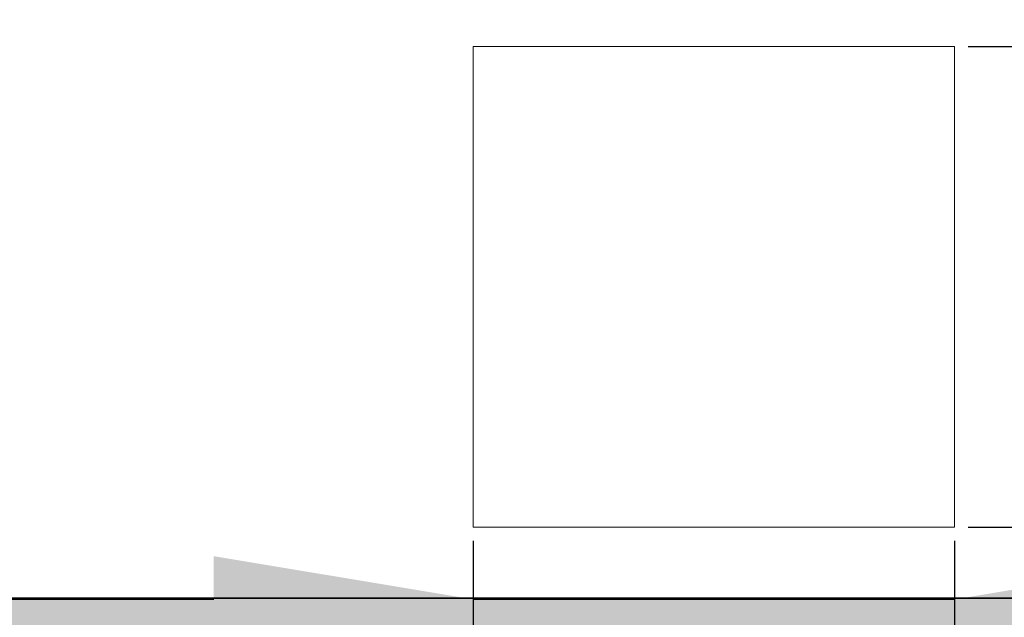
# Model space of a CAD drawing. Units: inches. Extents: x 2083 to 3317, y 1141 to 2115.
# Tile 238 of 256: x 3068 to 3114, y 1271 to 1299. Entities that reach past the tile are written whole.
import ezdxf

# ---------------------------------------------------------------- set-up
doc = ezdxf.new("R2010")
doc.units = ezdxf.units.IN
for name, color, linetype, lineweight in [('A-ANNO-DIMS', 2, 'Continuous', 18), ('A-FURN', 8, 'Continuous', 18), ('A-WALL', 7, 'Continuous', 35)]:
    doc.layers.add(name, color=color, linetype=linetype, lineweight=lineweight)
doc.layers.add('A-WALL-PATT', color=251, linetype='Continuous', lineweight=13, true_color=0x636466)
doc.styles.get("Standard").update_dxf_attribs({"font": 'arial.ttf'})
doc.dimstyles.new('ISO-25', dxfattribs={"dimtxt": 12, "dimasz": 12, "dimexe": 1.25, "dimexo": 0.625, "dimtad": 1, "dimlunit": 3, "dimtxsty": 'Standard', "dimcen": 2.5, "dimadec": 0, "dimazin": 0, "dimtfac": 1, "dimtmove": 0, "dimatfit": 3, "dimfxl": 1, "dimarcsym": 0})

# ---------------------------------------------------------------- blocks, each defined once
blk = doc.blocks.new('NIGHTSTAND-COMPACT')
blk.add_lwpolyline([(22.254, 22.255), (22.254, 0), (0, 0), (0, 22.255)], close=True)
blk = doc.blocks.new('*D26')
at = {"layer": 'A-ANNO-DIMS', "color": 0, "lineweight": -2, "transparency": 16777216}
for p, q in [((3088.986, 1274.915), (3088.986, 1270.952)), ((3111.24, 1274.915), (3111.24, 1270.952)), ((3076.986, 1272.202), (2840.262, 1272.202)), ((3111.24, 1272.202), (3088.986, 1272.202)), ((3123.24, 1272.202), (3135.24, 1272.202))]:
    blk.add_line(p, q, dxfattribs=at)
at = {"layer": 'A-ANNO-DIMS', "color": 0, "transparency": 16777216}
for points in [[(3076.986, 1274.202), (3076.986, 1270.202), (3088.986, 1272.202)], [(3123.24, 1274.202), (3123.24, 1270.202), (3111.24, 1272.202)]]:
    blk.add_solid(points, dxfattribs=at)
at = {"layer": 'Defpoints', "color": 0, "transparency": 16777216}
for p in [(3088.986, 1275.54), (3111.24, 1275.54), (3088.986, 1272.202)]:
    blk.add_point(p, dxfattribs=at)
at = {"layer": 'A-ANNO-DIMS', "color": 0, "transparency": 16777216, "insert": (2952.624, 1279.032), "char_height": 12, "attachment_point": 5}
blk.add_mtext('NIGHTSTAND 1\'-10 1/2" TYP.', dxfattribs=at)
blk = doc.blocks.new('*D27')
at = {"layer": 'A-ANNO-DIMS', "color": 0, "lineweight": -2, "transparency": 16777216}
for p, q in [((3114.578, 1309.794), (3114.578, 1321.794)), ((3111.865, 1297.794), (3115.828, 1297.794)), ((3114.578, 1297.794), (3114.578, 1275.54)), ((3111.865, 1275.54), (3115.828, 1275.54)), ((3114.578, 1263.54), (3114.578, 1140.989))]:
    blk.add_line(p, q, dxfattribs=at)
at = {"layer": 'A-ANNO-DIMS', "color": 0, "transparency": 16777216}
for points in [[(3112.578, 1309.794), (3116.578, 1309.794), (3114.578, 1297.794)], [(3112.578, 1263.54), (3116.578, 1263.54), (3114.578, 1275.54)]]:
    blk.add_solid(points, dxfattribs=at)
at = {"layer": 'Defpoints', "color": 0, "transparency": 16777216}
for p in [(3111.24, 1297.794), (3111.24, 1275.54), (3114.578, 1275.54)]:
    blk.add_point(p, dxfattribs=at)
at = {"layer": 'A-ANNO-DIMS', "color": 0, "transparency": 16777216, "insert": (3107.749, 1196.264), "char_height": 12, "attachment_point": 5, "rotation": 90}
blk.add_mtext('1\'-10 1/2" TYP.', dxfattribs=at)

msp = doc.modelspace()

# ---------------------------------------------------------------- hatches: boundary and pattern name
at = {"layer": 'A-WALL-PATT'}
h = msp.add_hatch(color=256, dxfattribs=at)
h.dxf.hatch_style = 1
h.paths.add_polyline_path([(3126.96, 2020.761), (2748.96, 2020.761), (2604.96, 2020.761), (2226.96, 2020.761), (2226.96, 1702.761), (2466.96, 1702.761), (2466.96, 1582.761), (2418.96, 1582.761), (2418.96, 1477.761), (2226.96, 1477.761), (2226.96, 1263.261), (2544.96, 1263.261), (2544.96, 1411.761), (2604.96, 1411.761), (2685.96, 1411.761), (2685.96, 1420.761), (2604.96, 1420.761), (2604.96, 1573.761), (2604.96, 1702.761), (2604.96, 2011.761), (2748.96, 2011.761), (2748.96, 1702.761), (2862.96, 1702.761), (2862.96, 1621.761), (2871.96, 1621.761), (2871.96, 1702.761), (2883.96, 1702.761), (2883.96, 1706.939, -0.026459), (2883.96, 1711.761), (2757.96, 1711.761), (2757.96, 1807.761), (2787.96, 1807.761), (2787.96, 1812.261), (2757.96, 1812.261), (2757.96, 2011.761), (2877.96, 2011.761), (2877.96, 1812.261), (2847.96, 1812.261), (2847.96, 1807.761), (2889.836, 1807.761), (2889.836, 1812.261), (2882.46, 1812.261), (2882.46, 2011.761), (3117.96, 2011.761), (3117.96, 1812.261), (2937.836, 1812.261), (2937.836, 1807.761), (2995.71, 1807.761), (2995.71, 1796.118), (3000.21, 1796.118), (3000.21, 1807.761), (3117.96, 1807.761), (3117.96, 1711.761), (3000.21, 1711.761), (3000.21, 1760.118), (2998.573, 1760.118, -0.020711), (2995.71, 1760.118), (2995.71, 1711.761), (2931.96, 1711.761), (2931.96, 1702.761), (3126.96, 1702.761)])
h.paths.add_polyline_path([(2471.46, 2011.761), (2471.46, 1810.011), (2462.717, 1810.011), (2462.717, 1805.511), (2505.96, 1805.511), (2505.96, 1810.011), (2475.96, 1810.011), (2475.96, 2011.761), (2595.96, 2011.761), (2595.96, 1810.011), (2565.96, 1810.011), (2565.96, 1805.511), (2595.96, 1805.511), (2595.96, 1711.761), (2235.96, 1711.761), (2235.96, 1805.511), (2353.71, 1805.511), (2353.71, 1796.054), (2358.21, 1796.054), (2358.21, 1805.511), (2414.717, 1805.511), (2414.717, 1810.011), (2235.96, 1810.011), (2235.96, 2011.761)], flags=16)
h.paths.add_polyline_path([(2270.205, 1994.61), (2270.205, 1970.61), (2246.205, 1970.61), (2246.205, 1994.61)], flags=0)
edge = h.paths.add_edge_path(flags=0)
edge.add_ellipse((2332.027, 1899.798), major_axis=(-3.043, 3.043), ratio=0.168252, start_angle=-161.3322, end_angle=-156.3071, ccw=False)
edge.add_ellipse((2333.082, 1898.744), major_axis=(-1.055, 1.055), ratio=0.453532, start_angle=-123.371, end_angle=-94.1591)
edge = h.paths.add_edge_path(flags=0)
edge.add_ellipse((2332.027, 1968.876), major_axis=(3.043, 3.043), ratio=0.168252, start_angle=18.6678, end_angle=23.6929)
edge.add_spline(control_points=[(2332.926, 1970.691), (2332.227, 1970.336), (2330.894, 1969.659), (2328.413, 1970.932), (2327.204, 1967.749), (2324.71, 1969.956), (2322.533, 1967.012), (2320.013, 1971.296), (2317.68, 1968.158), (2316.041, 1967.102), (2315.427, 1966.81)], knot_values=[0, 0, 0, 0, 2.267059, 4.324559, 6.685584, 8.878641, 11.121502, 14.300359, 17.755284, 19.732645, 19.732645, 19.732645, 19.732645], degree=3, periodic=0)
edge.add_ellipse((2332.027, 1968.876), major_axis=(3.043, 3.043), ratio=0.168252, start_angle=18.6678, end_angle=23.6929, ccw=False)
edge.add_ellipse((2333.082, 1969.931), major_axis=(1.055, 1.055), ratio=0.453532, start_angle=56.629, end_angle=85.8409, ccw=False)
edge = h.paths.add_edge_path(flags=0)
edge.add_spline(control_points=[(2296.428, 1967.988), (2293.628, 1965.336), (2287.704, 1959.727), (2299.744, 1949.996), (2294.533, 1935.669), (2290.573, 1920.604), (2293.394, 1909.974), (2296.185, 1904.967)], knot_values=[0.099185, 0.099185, 0.099185, 0.099185, 0.345301, 0.619822, 0.982653, 1.386093, 1.810555, 1.810555, 1.810555, 1.810555], degree=3, periodic=0)
edge.add_spline(control_points=[(2296.185, 1904.967), (2297.384, 1902.619), (2298.001, 1901.949), (2298.553, 1901.468)], knot_values=[0.006246, 0.006246, 0.006246, 0.006246, 0.055476, 0.055476, 0.055476, 0.055476], degree=3, periodic=0)
edge.add_spline(control_points=[(2298.553, 1901.468), (2297.259, 1900.923), (2295.225, 1900.232), (2293.06, 1900.614), (2292.101, 1900.788), (2292.09, 1900.791)], knot_values=[0.312835, 0.312835, 0.312835, 0.312835, 0.40178, 0.474987, 0.475903, 0.475903, 0.475903, 0.475903], degree=3, periodic=0)
edge.add_arc((2292.794, 1904.664), 3.937, 215.4209, 259.6982, ccw=False)
edge.add_spline(control_points=[(2289.585, 1902.382), (2289.477, 1902.535), (2289.368, 1902.688), (2289.261, 1902.841)], knot_values=[0.102872, 0.102872, 0.102872, 0.102872, 0.116896, 0.116896, 0.116896, 0.116896], degree=3, periodic=0)
edge.add_spline(control_points=[(2289.261, 1902.841), (2288.687, 1902.55), (2287.64, 1902.02), (2285.881, 1901.874), (2283.853, 1901.504), (2281.72, 1899.711), (2278.467, 1899.493), (2276.157, 1901.883), (2272.259, 1899.804), (2267.778, 1901.843), (2262.244, 1900.184), (2257.415, 1901.782), (2254.318, 1900.726), (2253.178, 1900.337)], knot_values=[0, 0, 0, 0, 1.907977, 3.477176, 5.261074, 7.972851, 11.680248, 13.717921, 16.939592, 22.789562, 27.502503, 33.595215, 37.145618, 37.145618, 37.145618, 37.145618], degree=3, periodic=0)
edge.add_line((2253.178, 1900.337), (2250.244, 1902.841))
edge.add_line((2250.244, 1902.841), (2250.244, 1965.833))
edge.add_line((2250.244, 1965.833), (2253.178, 1968.337))
edge.add_spline(control_points=[(2253.178, 1968.337), (2254.318, 1967.948), (2257.415, 1966.892), (2262.244, 1968.49), (2267.778, 1966.831), (2271.527, 1968.537), (2273.876, 1967.828), (2274.207, 1967.728)], knot_values=[0, 0, 0, 0, 0.09018, 0.244935, 0.364644, 0.513233, 0.537855, 0.537855, 0.537855, 0.537855], degree=3, periodic=0)
edge.add_arc((2274.353, 1963.793), 3.937, 72.0511, 92.1279, ccw=False)
edge.add_arc((2281.297, 1985.23), 18.596, 252.0511, 288.5657)
edge.add_arc((2292.317, 1956.029), 12.646, 71.0268, 113.7782, ccw=False)
edge = h.paths.add_edge_path(flags=0)
edge.add_spline(control_points=[(2274.899, 1951.856), (2275.066, 1951.617), (2275.233, 1951.377), (2275.398, 1951.136)], knot_values=[1.409916, 1.409916, 1.409916, 1.409916, 1.43159, 1.43159, 1.43159, 1.43159], degree=3, periodic=0)
edge.add_spline(control_points=[(2275.398, 1951.136), (2275.792, 1950.562), (2276.179, 1949.984), (2276.546, 1949.397)], knot_values=[1.358238, 1.358238, 1.358238, 1.358238, 1.409916, 1.409916, 1.409916, 1.409916], degree=3, periodic=0)
edge.add_line((2276.546, 1949.397), (2277.437, 1947.862))
edge.add_spline(control_points=[(2277.437, 1947.862), (2276.304, 1945.673), (2274.64, 1942.427), (2274.632, 1938.094), (2272.799, 1930.852), (2274.356, 1943.897), (2275.948, 1947.923), (2276.546, 1949.397)], knot_values=[0.005632, 0.005632, 0.005632, 0.005632, 0.186014, 0.266002, 0.357087, 0.59639, 0.739732, 0.739732, 0.739732, 0.739732], degree=3, periodic=0)
edge.add_spline(control_points=[(2276.546, 1949.397), (2276.179, 1949.984), (2275.792, 1950.562), (2275.398, 1951.136)], knot_values=[1.358238, 1.358238, 1.358238, 1.358238, 1.409916, 1.409916, 1.409916, 1.409916], degree=3, periodic=0)
edge.add_spline(control_points=[(2275.398, 1951.136), (2274.943, 1950.08), (2274.208, 1948.025), (2273.935, 1944.851), (2272.469, 1937.627), (2273.466, 1945.696), (2274.701, 1951.059), (2274.899, 1951.856)], knot_values=[0.104364, 0.104364, 0.104364, 0.104364, 0.189636, 0.269624, 0.36071, 0.600013, 0.644622, 0.644622, 0.644622, 0.644622], degree=3, periodic=0)
h.paths.add_polyline_path([(2269.168, 1963.128, -0.357527), (2268.171, 1960.976, -0.092561), (2268.171, 1939.436, -0.357527), (2269.168, 1937.285, -0.357527), (2267.016, 1938.282, -0.164785), (2254.686, 1938.282, -0.357527), (2252.534, 1937.285, -0.357527), (2253.531, 1939.436, -0.092561), (2253.531, 1960.976, -0.357527), (2252.534, 1963.128, -0.357527), (2254.686, 1962.131, -0.164785), (2267.016, 1962.131, -0.357527)], flags=0)
h.paths.add_polyline_path([(2248.874, 1967.802), (2248.874, 1957.028), (2249.458, 1957.028), (2249.458, 1911.647), (2248.874, 1911.647), (2248.874, 1900.873), (2246.512, 1900.873, 0.197327), (2244.15, 1902.457), (2244.15, 1966.218, 0.197327), (2246.512, 1967.802)], flags=0)
h.paths.add_polyline_path([(2269.168, 1931.389, -0.357527), (2268.171, 1929.238, -0.092561), (2268.171, 1907.698, -0.357527), (2269.168, 1905.547, -0.357527), (2267.016, 1906.544, -0.164785), (2254.686, 1906.544, -0.357527), (2252.534, 1905.547, -0.357527), (2253.531, 1907.698, -0.092561), (2253.531, 1929.238, -0.357527), (2252.534, 1931.389, -0.357527), (2254.686, 1930.392, -0.164785), (2267.016, 1930.392, -0.357527)], flags=0)
edge = h.paths.add_edge_path(flags=0)
edge.add_spline(control_points=[(2276.197, 1906.724), (2276.168, 1909.029), (2276.114, 1913.372), (2270.598, 1924.925), (2273.905, 1919.013), (2275.922, 1916.262), (2275.475, 1912.402), (2277.258, 1910.381), (2276.696, 1908.225), (2276.646, 1906.813), (2276.618, 1906.008)], knot_values=[0, 0, 0, 0, 8.61026, 16.221274, 18.843057, 23.804898, 27.440828, 29.356102, 31.203478, 33.650687, 33.650687, 33.650687, 33.650687], degree=3, periodic=0)
edge.add_spline(control_points=[(2276.618, 1906.008), (2276.623, 1905.624), (2276.498, 1904.629), (2275.442, 1903.855), (2274.937, 1903.08), (2274.859, 1902.841)], knot_values=[0.156488, 0.156488, 0.156488, 0.156488, 0.184398, 0.231376, 0.250598, 0.250598, 0.250598, 0.250598], degree=3, periodic=0)
edge.add_line((2274.859, 1902.841), (2276.506, 1902.841))
edge.add_spline(control_points=[(2276.506, 1902.841), (2276.788, 1903.085), (2277.665, 1904.125), (2278.25, 1904.341), (2277.654, 1908.527), (2278.156, 1906.228), (2278.1, 1905.286), (2278.847, 1904.069), (2277.857, 1903.415), (2277.874, 1902.991), (2277.904, 1902.841)], knot_values=[0.059574, 0.059574, 0.059574, 0.059574, 0.080753, 0.103741, 0.16972, 0.176036, 0.207137, 0.240474, 0.262341, 0.27366, 0.27366, 0.27366, 0.27366], degree=3, periodic=0)
edge.add_line((2277.904, 1902.841), (2280.03, 1902.841))
edge.add_spline(control_points=[(2280.03, 1902.841), (2279.888, 1903.088), (2279.499, 1903.982), (2280.152, 1905.939), (2278.104, 1909.658), (2279.762, 1907.185), (2280.328, 1904.875), (2280.485, 1903.49), (2281.463, 1903.249), (2281.758, 1902.936), (2281.834, 1902.841)], knot_values=[0.013856, 0.013856, 0.013856, 0.013856, 0.034874, 0.088867, 0.107879, 0.126738, 0.158714, 0.193757, 0.217487, 0.226722, 0.226722, 0.226722, 0.226722], degree=3, periodic=0)
edge.add_spline(control_points=[(2281.834, 1902.841), (2281.788, 1902.827), (2281.647, 1902.783), (2281.396, 1902.859), (2281.088, 1902.985), (2280.721, 1903.061), (2280.333, 1903.026), (2280.125, 1902.899), (2280.03, 1902.841)], knot_values=[0, 0, 0, 0, 0.14413, 0.435517, 0.749276, 1.153046, 1.548371, 1.878348, 1.878348, 1.878348, 1.878348], degree=3, periodic=0)
edge.add_line((2280.03, 1902.841), (2277.904, 1902.841))
edge.add_spline(control_points=[(2277.904, 1902.841), (2277.893, 1902.796), (2277.865, 1902.68), (2277.607, 1902.687), (2277.274, 1902.801), (2276.838, 1902.62), (2276.584, 1902.789), (2276.506, 1902.841)], knot_values=[0, 0, 0, 0, 0.127189, 0.326199, 0.628009, 1.24357, 1.515331, 1.515331, 1.515331, 1.515331], degree=3, periodic=0)
edge.add_line((2276.506, 1902.841), (2274.859, 1902.841))
edge.add_spline(control_points=[(2274.859, 1902.841), (2274.814, 1902.899), (2274.725, 1903.013), (2274.493, 1903.119), (2274.244, 1902.961), (2273.937, 1903.185), (2273.614, 1902.983), (2273.408, 1902.883), (2273.322, 1902.841)], knot_values=[0, 0, 0, 0, 0.21843, 0.436957, 0.687977, 0.990379, 1.398396, 1.69185, 1.69185, 1.69185, 1.69185], degree=3, periodic=0)
edge.add_spline(control_points=[(2273.322, 1902.841), (2273.617, 1903.446), (2274.274, 1904.538), (2276.027, 1904.574), (2276.207, 1906.584), (2276.197, 1906.724)], knot_values=[0.012227, 0.012227, 0.012227, 0.012227, 0.059472, 0.106218, 0.134458, 0.134458, 0.134458, 0.134458], degree=3, periodic=0)
h.paths.add_polyline_path([(2270.776, 1897.79), (2270.776, 1873.79), (2246.776, 1873.79), (2246.776, 1897.79)], flags=0)
h.paths.add_polyline_path([(2353.71, 1760.005), (2353.71, 1760.054), (2358.21, 1760.054, -0.033729)], flags=0)
h.paths.add_polyline_path([(2321.819, 1737.529), (2341.995, 1737.529, -0.414214), (2343.203, 1736.321), (2343.203, 1721.021, -0.414214), (2341.995, 1719.813), (2321.819, 1719.813, -0.414214), (2320.611, 1721.021), (2320.611, 1736.321, -0.414214)], flags=0)
h.paths.add_polyline_path([(2324.235, 1736.321), (2339.579, 1736.321, -0.414214), (2341.995, 1733.905), (2341.995, 1725.45, -0.414214), (2339.579, 1723.034), (2333.681, 1723.034), (2333.845, 1722.045, -0.870646), (2335.425, 1721.826, -0.767327), (2333.923, 1721.423), (2331.291, 1721.423, -0.767327), (2329.788, 1721.826, -0.870646), (2331.368, 1722.045), (2331.533, 1723.034), (2324.235, 1723.034, -0.414214), (2321.819, 1725.45), (2321.819, 1733.905, -0.414214)], flags=0)
h.paths.add_polyline_path([(2570.484, 1928.615), (2589.684, 1928.615), (2590.169, 1928.615), (2590.169, 1904.993), (2570.484, 1904.993)], flags=0)
h.paths.add_polyline_path([(2574.447, 1927.264, -1), (2572.829, 1927.264, -1)], flags=0)
h.paths.add_polyline_path([(2573.09, 1926.941), (2573.925, 1927.776), (2574.148, 1927.553), (2573.313, 1926.718)], flags=0)
h.paths.add_polyline_path([(2578.779, 1919.73, -1), (2571.592, 1919.73, -1)], flags=0)
h.paths.add_polyline_path([(2578.385, 1919.73, -1), (2571.985, 1919.73, -1)], flags=0)
h.paths.add_polyline_path([(2331.596, 1729.476, -1), (2333.618, 1729.476, -1)], flags=0)
h.paths.add_polyline_path([(2578.034, 1927.264, -1), (2576.416, 1927.264, -1)], flags=0)
h.paths.add_polyline_path([(2576.689, 1927.531), (2576.912, 1927.754), (2577.747, 1926.919), (2577.524, 1926.696)], flags=0)
h.paths.add_polyline_path([(2578.139, 1909.86, -1), (2572.232, 1909.86, -1)], flags=0)
h.paths.add_polyline_path([(2577.745, 1909.86, -1), (2572.625, 1909.86, -1)], flags=0)
h.paths.add_polyline_path([(2583.798, 1927.264, -1), (2582.179, 1927.264, -1)], flags=0)
h.paths.add_polyline_path([(2582.719, 1927.754), (2583.554, 1926.919), (2583.331, 1926.696), (2582.496, 1927.531)], flags=0)
h.paths.add_polyline_path([(2582.496, 1927.531), (2582.719, 1927.754), (2583.554, 1926.919), (2583.331, 1926.696)], flags=0)
h.paths.add_polyline_path([(2587.739, 1920.53, -1), (2581.832, 1920.53, -1)], flags=0)
h.paths.add_polyline_path([(2587.345, 1920.53, -1), (2582.225, 1920.53, -1)], flags=0)
h.paths.add_polyline_path([(2587.385, 1927.264, -1), (2585.766, 1927.264, -1)], flags=0)
h.paths.add_polyline_path([(2586.082, 1926.98), (2586.917, 1927.815), (2587.14, 1927.593), (2586.305, 1926.758)], flags=0)
h.paths.add_polyline_path([(2588.379, 1910.66, -1), (2581.192, 1910.66, -1)], flags=0)
h.paths.add_polyline_path([(2587.985, 1910.66, -1), (2581.585, 1910.66, -1)], flags=0)
h.paths.add_polyline_path([(2417.168, 1729.478), (2437.344, 1729.478, -0.414214), (2438.552, 1728.27), (2438.552, 1712.969, -0.414214), (2437.344, 1711.761), (2417.168, 1711.761, -0.414214), (2415.96, 1712.969), (2415.96, 1728.27, -0.414214)], flags=0)
h.paths.add_polyline_path([(2419.584, 1728.27), (2434.928, 1728.27, -0.414214), (2437.344, 1725.854), (2437.344, 1717.398, -0.414214), (2434.928, 1714.983), (2429.029, 1714.983), (2429.194, 1713.994, -0.870646), (2430.774, 1713.775, -0.767327), (2429.271, 1713.372), (2426.64, 1713.372, -0.767327), (2425.137, 1713.775, -0.870646), (2426.717, 1713.994), (2426.882, 1714.983), (2419.584, 1714.983, -0.414214), (2417.168, 1717.398), (2417.168, 1725.854, -0.414214)], flags=0)
h.paths.add_polyline_path([(2419.584, 1728.27), (2434.928, 1728.27, -0.414214), (2437.344, 1725.854), (2437.344, 1717.398, -0.414214), (2434.928, 1714.983), (2429.029, 1714.983), (2428.358, 1719.009), (2427.553, 1719.009), (2426.882, 1714.983), (2419.584, 1714.983, -0.414214), (2417.168, 1717.398), (2417.168, 1725.854, -0.414214)], flags=0)
h.paths.add_polyline_path([(2426.944, 1721.425, -1), (2428.967, 1721.425, -1)], flags=0)
h.paths.add_polyline_path([(2475.96, 1702.761), (2595.96, 1702.761), (2595.96, 1582.761), (2475.96, 1582.761)], flags=16)
h.paths.add_polyline_path([(2427.96, 1573.761), (2595.96, 1573.761), (2595.96, 1468.761), (2595.96, 1420.761), (2384.46, 1420.761), (2384.46, 1468.761), (2427.96, 1468.761)], flags=16)
h.paths.add_polyline_path([(2379.96, 1468.761), (2379.96, 1420.761), (2235.96, 1420.761), (2235.96, 1468.761)], flags=16)
h.paths.add_polyline_path([(2317.816, 1466.696), (2337.992, 1466.696, -0.414214), (2339.2, 1465.488), (2339.2, 1450.187, -0.414214), (2337.992, 1448.979), (2317.816, 1448.979, -0.414214), (2316.608, 1450.187), (2316.608, 1465.488, -0.414214)], flags=0)
h.paths.add_polyline_path([(2320.232, 1465.488), (2335.576, 1465.488, -0.414214), (2337.992, 1463.072), (2337.992, 1454.616, -0.414214), (2335.576, 1452.2), (2329.677, 1452.2), (2329.842, 1451.212, -0.870646), (2331.422, 1450.992, -0.767327), (2329.92, 1450.59), (2327.288, 1450.59, -0.767327), (2325.785, 1450.992, -0.870646), (2327.365, 1451.212), (2327.53, 1452.2), (2320.232, 1452.2, -0.414214), (2317.816, 1454.616), (2317.816, 1463.072, -0.414214)], flags=0)
h.paths.add_polyline_path([(2320.232, 1465.488), (2335.576, 1465.488, -0.414214), (2337.992, 1463.072), (2337.992, 1454.616, -0.414214), (2335.576, 1452.2), (2329.677, 1452.2), (2329.006, 1456.227), (2328.201, 1456.227), (2327.53, 1452.2), (2320.232, 1452.2, -0.414214), (2317.816, 1454.616), (2317.816, 1463.072, -0.414214)], flags=0)
h.paths.add_polyline_path([(2327.593, 1458.643, -1), (2329.615, 1458.643, -1)], flags=0)
h.paths.add_polyline_path([(2244.412, 1433.34), (2241.921, 1433.34, -0.414214), (2240.018, 1435.244), (2240.018, 1440.953, -0.414211), (2241.921, 1442.856), (2244.412, 1442.856, -1.976472)], flags=0)
h.paths.add_polyline_path([(2245.357, 1434.398, -0.414214), (2245.357, 1441.799, -2.144098)], flags=0)
h.paths.add_polyline_path([(2535.96, 1416.261), (2535.96, 1272.261), (2235.96, 1272.261), (2235.96, 1416.261)], flags=16)
h.paths.add_polyline_path([(2260.12, 1384.293), (2260.12, 1362.039), (2237.865, 1362.039), (2237.865, 1384.293)], flags=0)
edge = h.paths.add_edge_path(flags=0)
edge.add_line((2318.252, 1362.093), (2318.146, 1362.001))
edge.add_ellipse((2317.445, 1360.431), major_axis=(2.822, 2.822), ratio=0.168252, start_angle=18.6678, end_angle=20.9481, ccw=False)
edge.add_ellipse((2318.423, 1361.409), major_axis=(0.978, 0.978), ratio=0.453532, start_angle=56.629, end_angle=70.2262, ccw=False)
edge = h.paths.add_edge_path(flags=0)
edge.add_line((2319.107, 1295.571), (2319.015, 1295.677))
edge.add_ellipse((2317.445, 1296.378), major_axis=(-2.822, 2.822), ratio=0.168252, start_angle=-161.3322, end_angle=-159.0519, ccw=False)
edge.add_ellipse((2318.423, 1295.4), major_axis=(-0.978, 0.978), ratio=0.453532, start_angle=-123.371, end_angle=-109.7738)
edge = h.paths.add_edge_path(flags=0)
edge.add_spline(control_points=[(2284.21, 1301.17), (2284.581, 1300.445), (2284.891, 1299.892), (2285.16, 1299.461)], knot_values=[0.039066, 0.039066, 0.039066, 0.039066, 0.055476, 0.055476, 0.055476, 0.055476], degree=3, periodic=0)
edge.add_line((2285.16, 1299.461), (2284.21, 1301.17))
edge = h.paths.add_edge_path(flags=0)
edge.add_line((2280.412, 1297.298), (2283.37, 1297.036))
edge.add_line((2283.37, 1297.036), (2286.406, 1297.926))
edge.add_spline(control_points=[(2286.406, 1297.926), (2285.305, 1297.463), (2284.345, 1297.129), (2283.37, 1297.036)], knot_values=[0.394369, 0.394369, 0.394369, 0.394369, 0.475903, 0.475903, 0.475903, 0.475903], degree=3, periodic=0)
edge.add_spline(control_points=[(2283.37, 1297.036), (2283.281, 1297.028), (2282.316, 1296.957), (2281.313, 1297.134), (2280.423, 1297.296), (2280.412, 1297.298)], knot_values=[0.312835, 0.312835, 0.312835, 0.312835, 0.320246, 0.393453, 0.394369, 0.394369, 0.394369, 0.394369], degree=3, periodic=0)
edge = h.paths.add_edge_path(flags=0)
edge.add_line((2284.436, 1359.607), (2280.446, 1355.328))
edge.add_line((2280.446, 1355.328), (2279.58, 1351.018))
edge.add_line((2279.58, 1351.018), (2282.413, 1346.58))
edge.add_spline(control_points=[(2282.413, 1346.58), (2283.153, 1345.589), (2284.253, 1344.029), (2284.801, 1342.387), (2284.935, 1341.806)], knot_values=[1.240098, 1.240098, 1.240098, 1.240098, 1.332892, 1.382712, 1.382712, 1.382712, 1.382712], degree=3, periodic=0)
edge.add_spline(control_points=[(2284.935, 1341.806), (2285.319, 1340.141), (2285.233, 1338.409), (2284.91, 1336.654)], knot_values=[1.097484, 1.097484, 1.097484, 1.097484, 1.240098, 1.240098, 1.240098, 1.240098], degree=3, periodic=0)
edge.add_spline(control_points=[(2284.91, 1336.654), (2284.587, 1334.899), (2284.027, 1333.12), (2283.463, 1331.361)], knot_values=[0.95487, 0.95487, 0.95487, 0.95487, 1.097484, 1.097484, 1.097484, 1.097484], degree=3, periodic=0)
edge.add_line((2283.463, 1331.361), (2281.89, 1326.153))
edge.add_line((2281.89, 1326.153), (2280.756, 1321.056))
edge.add_line((2280.756, 1321.056), (2280.299, 1316.002))
edge.add_line((2280.299, 1316.002), (2280.716, 1310.95))
edge.add_line((2280.716, 1310.95), (2282.028, 1305.972))
edge.add_line((2282.028, 1305.972), (2284.21, 1301.17))
edge.add_spline(control_points=[(2284.21, 1301.17), (2283.341, 1302.73), (2282.612, 1304.336), (2282.028, 1305.972)], knot_values=[0.099185, 0.099185, 0.099185, 0.099185, 0.241799, 0.241799, 0.241799, 0.241799], degree=3, periodic=0)
edge.add_spline(control_points=[(2282.028, 1305.972), (2281.444, 1307.608), (2281.005, 1309.273), (2280.716, 1310.95)], knot_values=[0.241799, 0.241799, 0.241799, 0.241799, 0.384413, 0.384413, 0.384413, 0.384413], degree=3, periodic=0)
edge.add_spline(control_points=[(2280.716, 1310.95), (2280.433, 1312.588), (2280.289, 1314.277), (2280.299, 1315.962), (2280.299, 1316.002)], knot_values=[0.384413, 0.384413, 0.384413, 0.384413, 0.523647, 0.527028, 0.527028, 0.527028, 0.527028], degree=3, periodic=0)
edge.add_spline(control_points=[(2280.299, 1316.002), (2280.312, 1317.687), (2280.478, 1319.368), (2280.756, 1321.056)], knot_values=[0.527028, 0.527028, 0.527028, 0.527028, 0.669642, 0.669642, 0.669642, 0.669642], degree=3, periodic=0)
edge.add_spline(control_points=[(2280.756, 1321.056), (2281.035, 1322.744), (2281.426, 1324.44), (2281.89, 1326.153)], knot_values=[0.669642, 0.669642, 0.669642, 0.669642, 0.812256, 0.812256, 0.812256, 0.812256], degree=3, periodic=0)
edge.add_spline(control_points=[(2281.89, 1326.153), (2282.264, 1327.533), (2282.788, 1329.262), (2283.353, 1331.018), (2283.463, 1331.361)], knot_values=[0.812256, 0.812256, 0.812256, 0.812256, 0.927087, 0.95487, 0.95487, 0.95487, 0.95487], degree=3, periodic=0)
edge.add_line((2283.463, 1331.361), (2284.91, 1336.654))
edge.add_line((2284.91, 1336.654), (2284.935, 1341.806))
edge.add_line((2284.935, 1341.806), (2282.413, 1346.58))
edge.add_spline(control_points=[(2282.413, 1346.58), (2281.275, 1348.104), (2280.078, 1349.57), (2279.58, 1351.018)], knot_values=[1.382712, 1.382712, 1.382712, 1.382712, 1.525326, 1.525326, 1.525326, 1.525326], degree=3, periodic=0)
edge.add_spline(control_points=[(2279.58, 1351.018), (2279.443, 1351.415), (2279.136, 1352.857), (2279.735, 1354.29), (2280.446, 1355.328)], knot_values=[1.525326, 1.525326, 1.525326, 1.525326, 1.564439, 1.667941, 1.667941, 1.667941, 1.667941], degree=3, periodic=0)
edge.add_spline(control_points=[(2280.446, 1355.328), (2281.426, 1356.758), (2282.931, 1358.183), (2284.436, 1359.607)], knot_values=[1.667941, 1.667941, 1.667941, 1.667941, 1.810555, 1.810555, 1.810555, 1.810555], degree=3, periodic=0)
edge.add_arc((2280.623, 1348.518), 11.726, 71.0268, 113.7782)
edge.add_arc((2270.405, 1375.595), 17.244, 252.0511, 288.5657, ccw=False)
edge.add_arc((2263.966, 1355.718), 3.651, 72.0511, 92.1279)
edge.add_arc((2263.966, 1355.718), 3.651, 92.1279, 177.9851)
edge.add_spline(control_points=[(2260.318, 1355.846), (2260.26, 1354.221), (2260.551, 1350.187), (2262.999, 1346.766), (2264.473, 1344.649)], knot_values=[1.43159, 1.43159, 1.43159, 1.43159, 1.564144, 1.770695, 1.770695, 1.770695, 1.770695], degree=3, periodic=0)
edge.add_line((2264.473, 1344.649), (2264.936, 1343.983))
edge.add_spline(control_points=[(2263.801, 1340.248), (2263.843, 1340.514), (2264.067, 1341.756), (2264.513, 1343.002), (2264.935, 1343.981)], knot_values=[0.53657, 0.53657, 0.53657, 0.53657, 0.559349, 0.644622, 0.644622, 0.644622, 0.644622], degree=3, periodic=0)
edge.add_spline(control_points=[(2264.935, 1343.981), (2265.118, 1343.715), (2265.299, 1343.448), (2265.477, 1343.179)], knot_values=[1.384077, 1.384077, 1.384077, 1.384077, 1.409916, 1.409916, 1.409916, 1.409916], degree=3, periodic=0)
edge.add_spline(control_points=[(2265.477, 1343.179), (2265.655, 1342.911), (2265.829, 1342.641), (2265.999, 1342.369)], knot_values=[1.358238, 1.358238, 1.358238, 1.358238, 1.384077, 1.384077, 1.384077, 1.384077], degree=3, periodic=0)
edge.add_line((2265.999, 1342.369), (2266.826, 1340.946))
edge.add_spline(control_points=[(2266.826, 1340.946), (2268.894, 1337.09), (2271.398, 1325.843), (2270.516, 1310.569), (2275.919, 1301.861), (2277.79, 1299.199)], knot_values=[0.116896, 0.116896, 0.116896, 0.116896, 0.472987, 1.050969, 1.313793, 1.313793, 1.313793, 1.313793], degree=3, periodic=0)
edge.add_spline(control_points=[(2277.79, 1299.199), (2277.839, 1299.128), (2277.889, 1299.057), (2277.94, 1298.987)], knot_values=[0.109884, 0.109884, 0.109884, 0.109884, 0.116896, 0.116896, 0.116896, 0.116896], degree=3, periodic=0)
edge.add_line((2277.94, 1298.987), (2277.789, 1299.199))
edge.add_spline(control_points=[(2277.789, 1299.199), (2277.257, 1298.929), (2276.286, 1298.438), (2275.039, 1298.334), (2274.383, 1298.239), (2274.215, 1298.209)], knot_values=[33.12187, 33.12187, 33.12187, 33.12187, 35.029056, 36.598255, 37.144827, 37.144827, 37.144827, 37.144827], degree=3, periodic=0)
edge.add_line((2274.215, 1298.209), (2273.073, 1297.893))
edge.add_spline(control_points=[(2273.073, 1297.893), (2272.323, 1297.58), (2271.039, 1296.511), (2269.248, 1296.226), (2268.423, 1296.375)], knot_values=[26.532584, 26.532584, 26.532584, 26.532584, 29.198919, 31.839101, 31.839101, 31.839101, 31.839101], degree=3, periodic=0)
edge.add_line((2268.423, 1296.375), (2263.879, 1297.458))
edge.add_spline(control_points=[(2263.879, 1297.458), (2263.556, 1297.359), (2261.86, 1296.839), (2260.239, 1297.282), (2258.933, 1297.516)], knot_values=[15.919551, 15.919551, 15.919551, 15.919551, 16.939592, 21.226067, 21.226067, 21.226067, 21.226067], degree=3, periodic=0)
edge.add_line((2258.933, 1297.516), (2254.055, 1297.329))
edge.add_spline(control_points=[(2254.055, 1297.329), (2253.756, 1297.296), (2252.114, 1297.165), (2250.462, 1297.544), (2249.13, 1297.668)], knot_values=[5.306517, 5.306517, 5.306517, 5.306517, 6.276435, 10.613034, 10.613034, 10.613034, 10.613034], degree=3, periodic=0)
edge.add_line((2249.13, 1297.668), (2244.332, 1296.878))
edge.add_line((2244.332, 1296.878), (2241.611, 1299.199))
edge.add_line((2241.611, 1299.199), (2241.611, 1357.609))
edge.add_line((2241.611, 1357.609), (2244.332, 1359.931))
edge.add_line((2244.332, 1359.931), (2252.729, 1359.543))
edge.add_spline(control_points=[(2252.729, 1359.543), (2252.871, 1359.546), (2253.306, 1359.548), (2253.74, 1359.514), (2254.032, 1359.482)], knot_values=[0.233291, 0.233291, 0.233291, 0.233291, 0.244935, 0.268927, 0.268927, 0.268927, 0.268927], degree=3, periodic=0)
edge.add_line((2254.032, 1359.482), (2259.587, 1359.416))
edge.add_spline(control_points=[(2259.587, 1359.416), (2260.677, 1359.629), (2262.073, 1359.897), (2263.524, 1359.459), (2263.83, 1359.366)], knot_values=[0.422516, 0.422516, 0.422516, 0.422516, 0.513233, 0.537855, 0.537855, 0.537855, 0.537855], degree=3, periodic=0)
edge.add_arc((2263.966, 1355.718), 3.651, 72.0511, 92.1279, ccw=False)
edge.add_arc((2270.405, 1375.595), 17.244, 252.0511, 288.5657)
edge.add_arc((2280.623, 1348.518), 11.726, 71.0268, 113.7782, ccw=False)
h.paths.add_polyline_path([(2240.341, 1359.435), (2240.341, 1349.444), (2240.882, 1349.444), (2240.882, 1307.365), (2240.341, 1307.365), (2240.341, 1297.374), (2238.15, 1297.374, 0.197327), (2235.96, 1298.843), (2235.96, 1357.966, 0.197327), (2238.15, 1359.435)], flags=0)
h.paths.add_polyline_path([(2259.158, 1355.101, -0.357527), (2258.233, 1353.106, -0.092561), (2258.233, 1333.133, -0.357527), (2259.158, 1331.138, -0.357527), (2257.163, 1332.062, -0.164785), (2245.729, 1332.062, -0.357527), (2243.735, 1331.138, -0.357527), (2244.659, 1333.133, -0.092561), (2244.659, 1353.106, -0.357527), (2243.735, 1355.101, -0.357527), (2245.729, 1354.176, -0.164785), (2257.163, 1354.176, -0.357527)], flags=0)
edge = h.paths.add_edge_path(flags=0)
edge.add_line((2265.999, 1342.369), (2266.826, 1340.946))
edge.add_line((2266.826, 1340.946), (2265.308, 1337.814))
edge.add_line((2265.308, 1337.814), (2264.358, 1334.653))
edge.add_line((2264.358, 1334.653), (2264.262, 1333.8))
edge.add_spline(control_points=[(2264.262, 1333.8), (2264.208, 1333.187), (2264.162, 1332.366), (2264.007, 1331.414), (2263.969, 1331.202)], knot_values=[0.464444, 0.464444, 0.464444, 0.464444, 0.516691, 0.531608, 0.531608, 0.531608, 0.531608], degree=3, periodic=0)
edge.add_spline(control_points=[(2263.969, 1331.202), (2263.775, 1330.119), (2263.424, 1328.791), (2263.257, 1328.531), (2263.234, 1328.515)], knot_values=[0.372682, 0.372682, 0.372682, 0.372682, 0.44885, 0.464444, 0.464444, 0.464444, 0.464444], degree=3, periodic=0)
edge.add_spline(control_points=[(2263.234, 1328.515), (2263.096, 1328.42), (2263.131, 1329.301), (2263.275, 1330.616)], knot_values=[0.280919, 0.280919, 0.280919, 0.280919, 0.372682, 0.372682, 0.372682, 0.372682], degree=3, periodic=0)
edge.add_spline(control_points=[(2263.275, 1330.616), (2263.419, 1331.93), (2263.672, 1333.677), (2263.97, 1335.315)], knot_values=[0.189157, 0.189157, 0.189157, 0.189157, 0.280919, 0.280919, 0.280919, 0.280919], degree=3, periodic=0)
edge.add_spline(control_points=[(2263.97, 1335.315), (2264.1, 1336.032), (2264.419, 1337.622), (2264.755, 1338.864), (2264.947, 1339.491)], knot_values=[0.097394, 0.097394, 0.097394, 0.097394, 0.137578, 0.189157, 0.189157, 0.189157, 0.189157], degree=3, periodic=0)
edge.add_spline(control_points=[(2264.947, 1339.491), (2265.29, 1340.606), (2265.644, 1341.494), (2265.999, 1342.369)], knot_values=[0.005632, 0.005632, 0.005632, 0.005632, 0.097394, 0.097394, 0.097394, 0.097394], degree=3, periodic=0)
h.paths.add_polyline_path([(2259.158, 1325.671, -0.357527), (2258.233, 1323.676, -0.092561), (2258.233, 1303.703, -0.357527), (2259.158, 1301.708, -0.357527), (2257.163, 1302.633, -0.164785), (2245.729, 1302.633, -0.357527), (2243.735, 1301.708, -0.357527), (2244.659, 1303.703, -0.092561), (2244.659, 1323.676, -0.357527), (2243.735, 1325.671, -0.357527), (2245.729, 1324.747, -0.164785), (2257.163, 1324.747, -0.357527)], flags=0)
edge = h.paths.add_edge_path(flags=0)
edge.add_spline(control_points=[(2261.709, 1317.311), (2261.679, 1317.418), (2261.762, 1317.389), (2262.491, 1316.09), (2262.962, 1315.301)], knot_values=[14.955861, 14.955861, 14.955861, 14.955861, 16.221274, 18.694826, 18.694826, 18.694826, 18.694826], degree=3, periodic=0)
edge.add_spline(control_points=[(2262.962, 1315.301), (2262.99, 1315.254), (2263.702, 1314.067), (2264.349, 1313.127), (2264.73, 1312.164)], knot_values=[18.694826, 18.694826, 18.694826, 18.694826, 18.843057, 22.433791, 22.433791, 22.433791, 22.433791], degree=3, periodic=0)
edge.add_spline(control_points=[(2264.73, 1312.164), (2264.876, 1311.796), (2265.177, 1310.77), (2265.143, 1309.559), (2265.248, 1308.824)], knot_values=[22.433791, 22.433791, 22.433791, 22.433791, 23.804898, 26.172756, 26.172756, 26.172756, 26.172756], degree=3, periodic=0)
edge.add_line((2265.248, 1308.824), (2265.851, 1307.172))
edge.add_spline(control_points=[(2265.851, 1307.172), (2266.065, 1306.822), (2266.384, 1306.332), (2266.424, 1305.781), (2266.42, 1305.611)], knot_values=[28.062562, 28.062562, 28.062562, 28.062562, 29.356102, 29.911721, 29.911721, 29.911721, 29.911721], degree=3, periodic=0)
edge.add_spline(control_points=[(2266.42, 1305.611), (2266.416, 1305.433), (2266.394, 1305.25), (2266.365, 1305.066)], knot_values=[29.911721, 29.911721, 29.911721, 29.911721, 30.497837, 30.497837, 30.497837, 30.497837], degree=3, periodic=0)
edge.add_line((2266.365, 1305.066), (2266.066, 1302.136))
edge.add_spline(control_points=[(2266.066, 1302.136), (2266.071, 1301.78), (2265.998, 1301.2), (2265.663, 1300.759), (2265.509, 1300.586)], knot_values=[0.156488, 0.156488, 0.156488, 0.156488, 0.184398, 0.203543, 0.203543, 0.203543, 0.203543], degree=3, periodic=0)
edge.add_line((2265.509, 1300.586), (2264.435, 1299.199))
edge.add_line((2264.435, 1299.199), (2265.962, 1299.199))
edge.add_line((2265.962, 1299.199), (2267.336, 1301.175))
edge.add_line((2267.336, 1301.175), (2267.312, 1301.986))
edge.add_spline(control_points=[(2267.312, 1301.986), (2267.261, 1302.862), (2267.16, 1303.737), (2267.271, 1303.326)], knot_values=[0.126229, 0.126229, 0.126229, 0.126229, 0.166617, 0.166617, 0.166617, 0.166617], degree=3, periodic=0)
edge.add_spline(control_points=[(2267.271, 1303.326), (2267.28, 1303.294), (2267.31, 1303.175), (2267.373, 1302.884), (2267.406, 1302.683), (2267.418, 1302.601)], knot_values=[0.166617, 0.166617, 0.166617, 0.166617, 0.16972, 0.176036, 0.180765, 0.180765, 0.180765, 0.180765], degree=3, periodic=0)
edge.add_spline(control_points=[(2267.744, 1300.988), (2267.688, 1301.151), (2267.481, 1301.657), (2267.484, 1302.145), (2267.418, 1302.601)], knot_values=[0.180765, 0.180765, 0.180765, 0.180765, 0.193767, 0.220139, 0.220139, 0.220139, 0.220139], degree=3, periodic=0)
edge.add_line((2267.418, 1302.601), (2267.744, 1300.988))
edge.add_spline(control_points=[(2267.744, 1300.988), (2267.832, 1300.732), (2267.932, 1300.31), (2267.555, 1299.975), (2267.429, 1299.829)], knot_values=[0.220139, 0.220139, 0.220139, 0.220139, 0.240474, 0.25489, 0.25489, 0.25489, 0.25489], degree=3, periodic=0)
edge.add_line((2267.429, 1299.829), (2267.258, 1299.199))
edge.add_line((2267.258, 1299.199), (2269.23, 1299.199))
edge.add_spline(control_points=[(2269.23, 1299.199), (2269.099, 1299.429), (2268.843, 1300.016), (2269.012, 1300.916), (2268.947, 1301.661)], knot_values=[0.013856, 0.013856, 0.013856, 0.013856, 0.034874, 0.067073, 0.067073, 0.067073, 0.067073], degree=3, periodic=0)
edge.add_line((2268.947, 1301.661), (2268.432, 1303.603))
edge.add_spline(control_points=[(2268.432, 1303.603), (2268.176, 1304.192), (2267.596, 1305.251), (2268.041, 1304.623), (2268.251, 1304.282)], knot_values=[0.090155, 0.090155, 0.090155, 0.090155, 0.107879, 0.120289, 0.120289, 0.120289, 0.120289], degree=3, periodic=0)
edge.add_spline(control_points=[(2268.251, 1304.282), (2268.361, 1304.105), (2269.058, 1302.918), (2269.383, 1301.59), (2269.521, 1300.776), (2269.575, 1300.556)], knot_values=[0.120289, 0.120289, 0.120289, 0.120289, 0.126738, 0.158714, 0.173506, 0.173506, 0.173506, 0.173506], degree=3, periodic=0)
edge.add_line((2269.575, 1300.556), (2270.686, 1299.421))
edge.add_spline(control_points=[(2270.686, 1299.421), (2270.767, 1299.357), (2270.838, 1299.281), (2270.903, 1299.199)], knot_values=[0.21816, 0.21816, 0.21816, 0.21816, 0.226722, 0.226722, 0.226722, 0.226722], degree=3, periodic=0)
edge.add_line((2270.937, 1299.193), (2270.903, 1299.199))
edge.add_spline(control_points=[(2270.903, 1299.199), (2270.86, 1299.186), (2270.73, 1299.146), (2270.496, 1299.216), (2270.272, 1299.308), (2270.121, 1299.348), (2270.063, 1299.36)], knot_values=[0.939174, 0.939174, 0.939174, 0.939174, 1.083304, 1.374691, 1.68845, 1.878348, 1.878348, 1.878348, 1.878348], degree=3, periodic=0)
edge.add_line((2270.063, 1299.36), (2269.23, 1299.199))
edge.add_line((2269.23, 1299.199), (2267.258, 1299.199))
edge.add_spline(control_points=[(2267.258, 1299.199), (2267.248, 1299.157), (2267.223, 1299.05), (2266.984, 1299.057), (2266.809, 1299.116), (2266.677, 1299.109), (2266.637, 1299.105)], knot_values=[0.757665, 0.757665, 0.757665, 0.757665, 0.884854, 1.083864, 1.385675, 1.515331, 1.515331, 1.515331, 1.515331], degree=3, periodic=0)
edge.add_spline(control_points=[(2266.637, 1299.105), (2266.485, 1299.089), (2266.236, 1299.017), (2266.035, 1299.151), (2265.962, 1299.199)], knot_values=[0, 0, 0, 0, 0.485905, 0.757665, 0.757665, 0.757665, 0.757665], degree=3, periodic=0)
edge.add_line((2265.962, 1299.199), (2264.435, 1299.199))
edge.add_line((2264.435, 1299.199), (2263.858, 1299.367))
edge.add_spline(control_points=[(2263.858, 1299.367), (2263.819, 1299.371), (2263.78, 1299.386), (2263.74, 1299.402)], knot_values=[0.845925, 0.845925, 0.845925, 0.845925, 0.978627, 0.978627, 0.978627, 0.978627], degree=3, periodic=0)
edge.add_line((2263.722, 1299.396), (2263.01, 1299.199))
edge.add_spline(control_points=[(2263.01, 1299.199), (2263.246, 1299.683), (2263.506, 1300.128), (2263.873, 1300.408)], knot_values=[0.012227, 0.012227, 0.012227, 0.012227, 0.052971, 0.052971, 0.052971, 0.052971], degree=3, periodic=0)
edge.add_spline(control_points=[(2263.873, 1300.408), (2263.932, 1300.453), (2264.084, 1300.553), (2264.255, 1300.624), (2264.36, 1300.665)], knot_values=[0.052971, 0.052971, 0.052971, 0.052971, 0.059472, 0.069086, 0.069086, 0.069086, 0.069086], degree=3, periodic=0)
edge.add_line((2264.36, 1300.665), (2265.142, 1301.078))
edge.add_line((2265.142, 1301.078), (2265.676, 1302.8))
edge.add_line((2265.676, 1302.8), (2265.541, 1305.704))
edge.add_line((2265.541, 1305.704), (2264.803, 1309.328))
edge.add_line((2264.803, 1309.328), (2263.041, 1314.092))
edge.add_spline(control_points=[(2263.041, 1314.092), (2262.384, 1315.671), (2261.796, 1316.998), (2261.709, 1317.311)], knot_values=[11.216896, 11.216896, 11.216896, 11.216896, 14.955861, 14.955861, 14.955861, 14.955861], degree=3, periodic=0)
h.paths.add_polyline_path([(2871.96, 1416.261), (2895.91, 1416.261), (2895.91, 1420.761), (2871.96, 1420.761), (2871.96, 1501.761), (2862.96, 1501.761), (2862.96, 1420.761), (2805.96, 1420.761), (2805.96, 1411.761), (2862.96, 1411.761), (2862.96, 1263.261), (3126.96, 1263.261), (3126.96, 1411.761), (3126.96, 1486.761), (2943.96, 1486.761), (2943.96, 1477.761), (2967.86, 1477.761), (2967.86, 1420.761), (2943.91, 1420.761), (2943.91, 1416.261), (3117.96, 1416.261), (3117.96, 1420.761), (2972.36, 1420.761), (2972.36, 1477.761), (3117.96, 1477.761), (3117.96, 1420.761), (3117.96, 1272.261), (2871.96, 1272.261)], flags=0)
h.paths.add_polyline_path([(2457.126, 1485.943), (2527.603, 1485.943), (2527.603, 1537.636), (2457.126, 1537.636)], flags=8)
h.paths.add_polyline_path([(2481.005, 1609.982), (2590.766, 1609.982), (2590.766, 1682.003), (2481.005, 1682.003)], flags=8)
h.paths.add_polyline_path([(2483.085, 1729.127), (2553.562, 1729.127), (2553.562, 1780.82), (2483.085, 1780.82)], flags=8)
h = msp.add_hatch(color=256, dxfattribs=at)
h.dxf.hatch_style = 1
h.paths.add_polyline_path([(3126.96, 1486.761), (2943.96, 1486.761), (2943.96, 1477.761), (2967.86, 1477.761), (2967.86, 1420.761), (2943.91, 1420.761), (2943.91, 1416.261), (3117.96, 1416.261), (3117.96, 1420.761), (2972.36, 1420.761), (2972.36, 1477.761), (3117.96, 1477.761), (3117.96, 1420.761), (3117.96, 1272.261), (2871.96, 1272.261), (2871.96, 1416.261), (2895.91, 1416.261), (2895.91, 1420.761), (2871.96, 1420.761), (2871.96, 1501.761), (2862.96, 1501.761), (2862.96, 1420.761), (2805.96, 1420.761), (2805.96, 1411.761), (2862.96, 1411.761), (2862.96, 1263.261), (3126.96, 1263.261), (3126.96, 1411.761)])

# ---------------------------------------------------------------- linework, layer by layer
at = {"layer": 'A-WALL'}
msp.add_line((2871.96, 1272.261), (3117.96, 1272.261), dxfattribs=at)

# ---------------------------------------------------------------- block references
at = {"layer": 'A-FURN', "rotation": 180}
msp.add_blockref('NIGHTSTAND-COMPACT', (3111.24, 1297.795), dxfattribs=at)

# ---------------------------------------------------------------- dimensions: what is measured, and where the dimension line sits
at = {"layer": 'A-ANNO-DIMS'}
for base, p1, p2, angle, text, picture, middle in [((3114.578, 1275.54), (3111.24, 1297.794), (3111.24, 1275.54), 270, '<> TYP.', '*D27', (3107.749, 1196.264)), ((3088.986, 1272.202), (3111.24, 1275.54), (3088.986, 1275.54), 180, 'NIGHTSTAND <> TYP.', '*D26', (2952.624, 1279.032))]:
    dim = msp.add_linear_dim(base=base, p1=p1, p2=p2, angle=angle, text=text, dimstyle='ISO-25', override={"dimdec": 1, "dimlfac": 1, "dimrnd": 0, "dimzin": 1, "dimdsep": 46, "dimlunit": 4, "dimfrac": 2}, dxfattribs=at)
    dim.commit()
    dim.dimension.update_dxf_attribs({"geometry": picture, "text_midpoint": middle})

doc.saveas('drawing.dxf')
